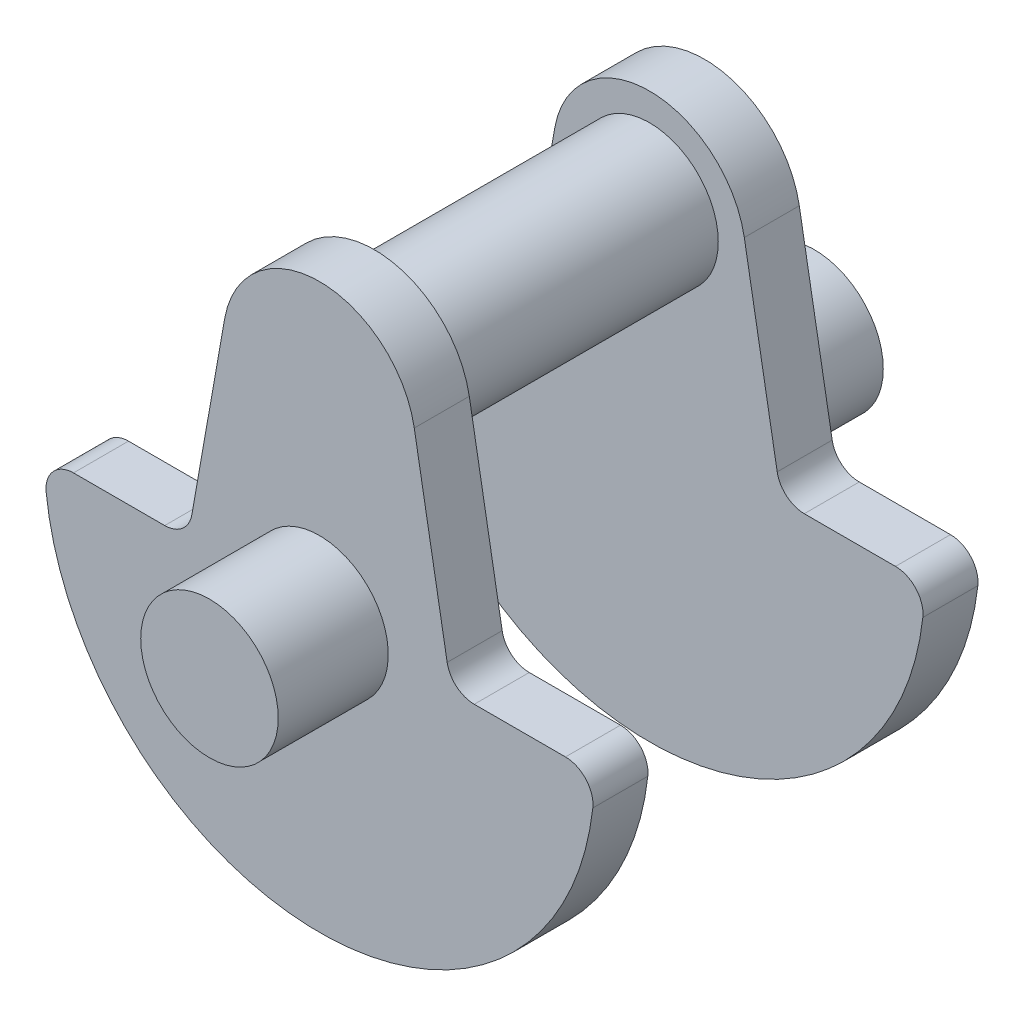
from build123d import *

# Parameters (mm, degrees)
CRANK_WEB_DEPTH       = 10
SKETCH1_4_R           = 12.5
MAIN_JOURNAL_DEPTH    = 30
CRANK_PIN_SKETCH_25_R = 12.5
CRANK_PIN_25_DEPTH    = 50


with BuildPart() as part:
    # Crank Web Profile → Crank Web (new body)
    with BuildSketch(Plane.XY):
        with BuildLine():
            Line((-28.136908189, 0), (-44.72135955, 0))
            ThreePointArc((-44.72135955, 0), (-48.448139512, -1.666666667), (-49.6903995, -5.555555556))
            ThreePointArc((-49.6903995, -5.555555556), (0, -50), (49.6903995, -5.555555556))
            ThreePointArc((49.6903995, -5.555555556), (48.448139512, -1.666666667), (44.72135955, 0))
            Line((44.72135955, 0), (28.136908189, 0))
            ThreePointArc((28.136908189, 0), (24.92297014, 1.169777784), (23.212869424, 4.131759112))
            Line((23.212869424, 4.131759112), (17.234135678, 38.038843109))
            ThreePointArc((17.234135678, 38.038843109), (0, 52.5), (-17.234135678, 38.038843109))
            Line((-17.234135678, 38.038843109), (-23.212869424, 4.131759112))
            ThreePointArc((-23.212869424, 4.131759112), (-24.92297014, 1.169777784), (-28.136908189, 0))
        make_face()
    crank_web = extrude(amount=-CRANK_WEB_DEPTH)

    # Sketch1_4 → Main Journal (add)
    with BuildSketch(Plane.XY):
        Circle(SKETCH1_4_R)
    main_journal = extrude(amount=-MAIN_JOURNAL_DEPTH)

    # Crank Pin Sketch _25 → Crank Pin _25 (add)
    with BuildSketch(Plane.XY):
        with Locations((0, 35)):
            Circle(CRANK_PIN_SKETCH_25_R)
    extrude(amount=CRANK_PIN_25_DEPTH)

    # Mirror Web and Journal: Crank Web, Main Journal across plane
    add(crank_web.mirror(Plane.XY.offset(25)))
    add(main_journal.mirror(Plane.XY.offset(25)))


solid = part.part
